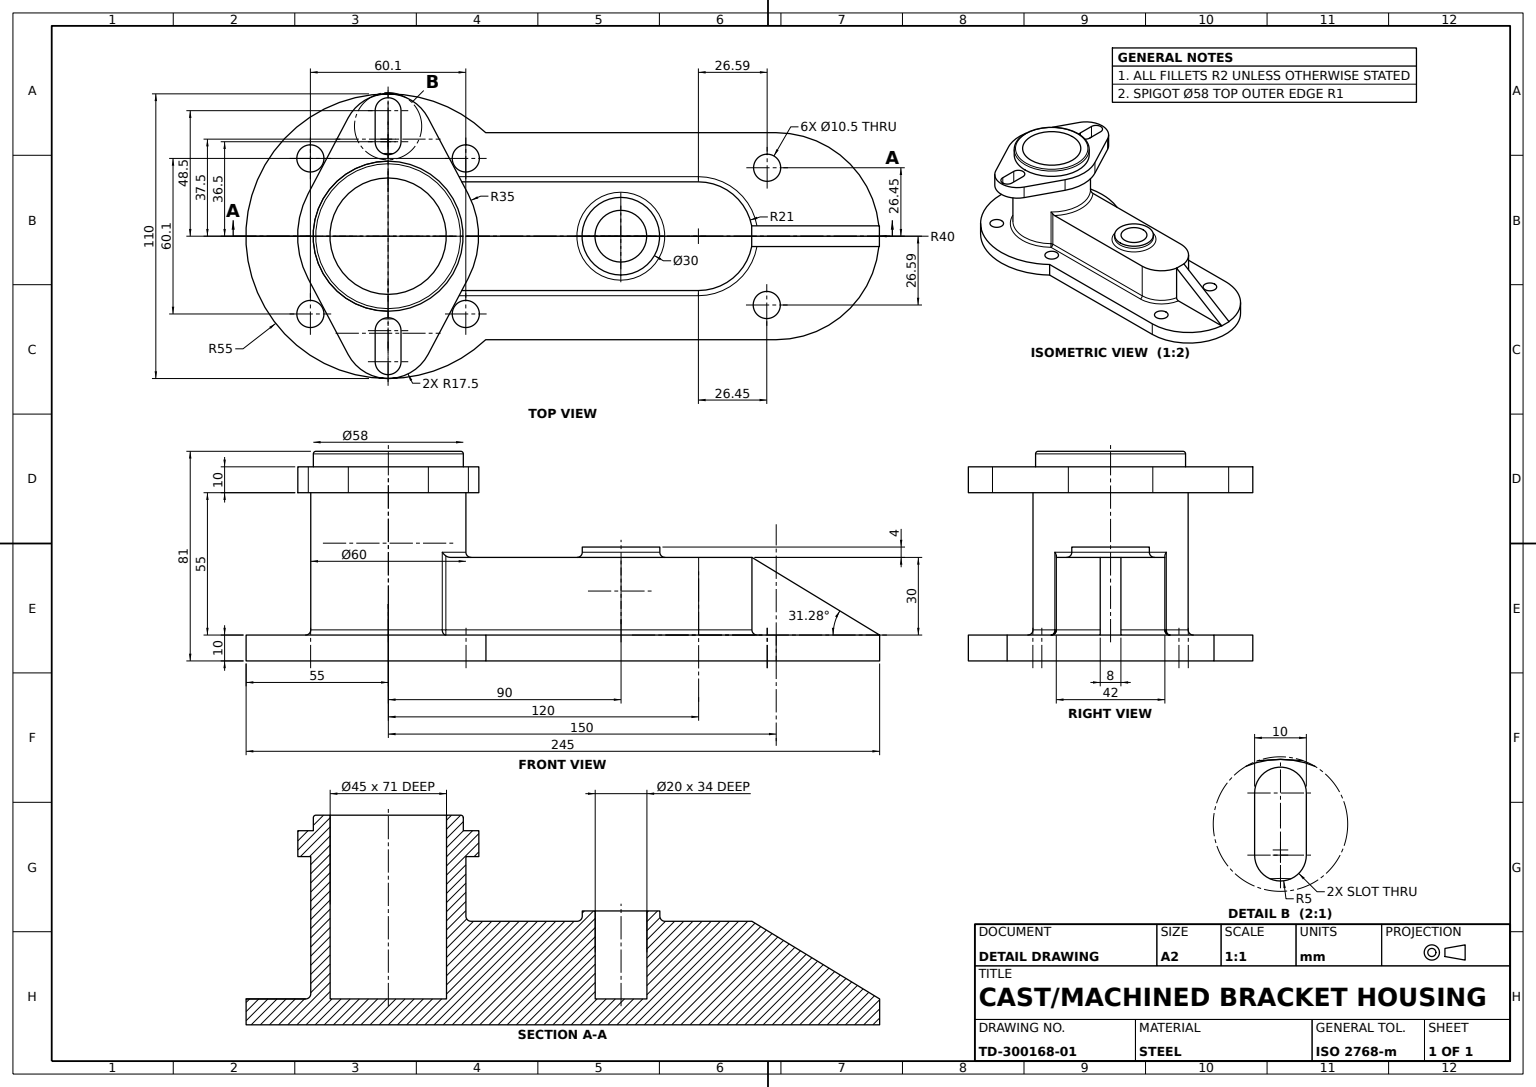
from build123d import *

# Parameters (mm, degrees)
BASE_PLATE_DEPTH                  = 10
BEARING_COLUMN_SKETCH_R           = 30
BEARING_COLUMN_60_DEPTH           = 55
TOP_FLANGE_DEPTH                  = 10
BEARING_SPIGOT_SKETCH_R           = 29
BEARING_SPIGOT_58_DEPTH           = 6
BEARING_BORE_SKETCH_R             = 22.5
BEARING_BORE_45_DEPTH             = 61
FLANGE_SLOTS_2X_DEPTH             = 10
ARM_BLOCK_DEPTH                   = 30
COLUMN_CLEARANCE_SKETCH_R         = 22.5
COLUMN_CLEARANCE_CUT_45_DEPTH     = 30
ARM_BOSS_SKETCH_R                 = 15
ARM_BOSS_30_DEPTH                 = 4
ARM_BOSS_BORE_SKETCH_R            = 10
ARM_BOSS_BORE_20_DEPTH            = 34
BASE_MOUNTING_HOLES_SKETCH_R      = 5.25
BASE_MOUNTING_HOLES_4X_10_5_DEPTH = 34
BASE_DIAGONAL_HOLES_SKETCH_R      = 5.25
BASE_DIAGONAL_HOLES_2X_10_5_DEPTH = 34
GUSSET_RIB_SKETCH_W               = 8
GUSSET_RIB_SKETCH_H               = 30
GUSSET_RIB_DEPTH                  = 50
RIB_TRIM_CUT_DEPTH                = 215.80689002
RIB_TRIM_CUT_DEPTH_BACK           = 49.8
COLUMN_ARM_FILLET_R2_R            = 2
COLUMN_BASE_FILLET_R2_R           = 2
ARM_BOSS_FILLET_R2_R              = 2
SPIGOT_FILLET_R1_R                = 1


with BuildPart() as part:
    # Base Plate Sketch → Base Plate (new body)
    with BuildSketch(Plane(origin=(0, 0, 0), x_dir=(1, 0, 0), z_dir=(0, 1, 0))):
        with BuildLine():
            Line((37.749172176, 40), (150, 40))
            ThreePointArc((150, 40), (190, 0), (150, -40))
            Line((150, -40), (37.749172176, -40))
            ThreePointArc((37.749172176, -40), (-55, 0), (37.749172176, 40))
        make_face()
    extrude(amount=BASE_PLATE_DEPTH)

    # Bearing Column Sketch → Bearing Column Ø60 (add)
    with BuildSketch(Plane(origin=(0, 10, 0), x_dir=(1, 0, 0), z_dir=(0, 1, 0))):
        with Locations(Location((0, 0, 0), (0, 0, 270))):
            Circle(BEARING_COLUMN_SKETCH_R)
    extrude(amount=BEARING_COLUMN_60_DEPTH)

    # Top Flange Sketch → Top Flange (add)
    with BuildSketch(Plane(origin=(0, 65, 0), x_dir=(1, 0, 0), z_dir=(0, 1, 0))):
        with BuildLine():
            Line((-15.477582355, 45.666666667), (-30.95516471, 16.333333333))
            ThreePointArc((-30.95516471, 16.333333333), (-35, 0), (-30.95516471, -16.333333333))
            Line((-30.95516471, -16.333333333), (-15.477582355, -45.666666667))
            ThreePointArc((-15.477582355, -45.666666667), (0, -55), (15.477582355, -45.666666667))
            Line((15.477582355, -45.666666667), (30.95516471, -16.333333333))
            ThreePointArc((30.95516471, -16.333333333), (35, 0), (30.95516471, 16.333333333))
            Line((30.95516471, 16.333333333), (15.477582355, 45.666666667))
            ThreePointArc((15.477582355, 45.666666667), (0, 55), (-15.477582355, 45.666666667))
        make_face()
    extrude(amount=TOP_FLANGE_DEPTH)

    # Bearing Spigot Sketch → Bearing Spigot Ø58 (add)
    with BuildSketch(Plane(origin=(0, 75, 0), x_dir=(1, 0, 0), z_dir=(0, 1, 0))):
        with Locations(Location((0, 0, 0), (0, 0, 270))):
            Circle(BEARING_SPIGOT_SKETCH_R)
    extrude(amount=BEARING_SPIGOT_58_DEPTH)

    # Bearing Bore Sketch → Bearing Bore Ø45 (cut)
    with BuildSketch(Plane(origin=(0, 81, 0), x_dir=(1, 0, 0), z_dir=(0, 1, 0))):
        with Locations(Location((0, 0, 0), (0, 0, 270))):
            Circle(BEARING_BORE_SKETCH_R)
    extrude(amount=-BEARING_BORE_45_DEPTH, mode=Mode.SUBTRACT)

    # Flange Slots Sketch → Flange Slots 2x (cut)
    with BuildSketch(Plane(origin=(0, 75, 0), x_dir=(1, 0, 0), z_dir=(0, 1, 0))):
        with BuildLine():
            Line((-5, 36.5), (-5, 48.5))
            ThreePointArc((-5, 48.5), (0, 53.5), (5, 48.5))
            Line((5, 48.5), (5, 36.5))
            ThreePointArc((5, 36.5), (0, 31.5), (-5, 36.5))
        make_face()
        with BuildLine():
            Line((5, -36.5), (5, -48.5))
            ThreePointArc((5, -48.5), (0, -53.5), (-5, -48.5))
            Line((-5, -48.5), (-5, -36.5))
            ThreePointArc((-5, -36.5), (0, -31.5), (5, -36.5))
        make_face()
    extrude(amount=-FLANGE_SLOTS_2X_DEPTH, mode=Mode.SUBTRACT)

    # Arm Block Sketch → Arm Block (add)
    with BuildSketch(Plane(origin=(0, 10, 0), x_dir=(1, 0, 0), z_dir=(0, 1, 0))):
        with BuildLine():
            Line((120, 21), (20, 21))
            Line((20, 21), (20, -21))
            Line((20, -21), (120, -21))
            ThreePointArc((120, -21), (141, 0), (120, 21))
        make_face()
    extrude(amount=ARM_BLOCK_DEPTH)

    # Column Clearance Sketch → Column Clearance Cut Ø45 (cut)
    with BuildSketch(Plane(origin=(0, 40, 0), x_dir=(1, 0, 0), z_dir=(0, 1, 0))):
        with Locations(Location((0, 0, 0), (0, 0, 270))):
            Circle(COLUMN_CLEARANCE_SKETCH_R)
    extrude(amount=-COLUMN_CLEARANCE_CUT_45_DEPTH, mode=Mode.SUBTRACT)

    # Arm Boss Sketch → Arm Boss Ø30 (add)
    with BuildSketch(Plane(origin=(0, 40, 0), x_dir=(1, 0, 0), z_dir=(0, 1, 0))):
        with Locations(Location((90, 0, 0), (0, 0, 270))):
            Circle(ARM_BOSS_SKETCH_R)
    extrude(amount=ARM_BOSS_30_DEPTH)

    # Arm Boss Bore Sketch → Arm Boss Bore Ø20 (cut)
    with BuildSketch(Plane(origin=(0, 44, 0), x_dir=(1, 0, 0), z_dir=(0, 1, 0))):
        with Locations(Location((90, 0, 0), (0, 0, 270))):
            Circle(ARM_BOSS_BORE_SKETCH_R)
    extrude(amount=-ARM_BOSS_BORE_20_DEPTH, mode=Mode.SUBTRACT)

    # Base Mounting Holes Sketch → Base Mounting Holes 4xØ10.5 (cut)
    with BuildSketch(Plane(origin=(0, 10, 0), x_dir=(1, 0, 0), z_dir=(0, 1, 0))):
        with Locations(Location((-30.0520382, 30.0520382, 0), (0, 0, 270))):
            Circle(BASE_MOUNTING_HOLES_SKETCH_R)
        with Locations(Location((30.0520382, 30.0520382, 0), (0, 0, 270))):
            Circle(BASE_MOUNTING_HOLES_SKETCH_R)
        with Locations(Location((30.0520382, -30.0520382, 0), (0, 0, 270))):
            Circle(BASE_MOUNTING_HOLES_SKETCH_R)
        with Locations(Location((-30.0520382, -30.0520382, 0), (0, 0, 270))):
            Circle(BASE_MOUNTING_HOLES_SKETCH_R)
    extrude(amount=-BASE_MOUNTING_HOLES_4X_10_5_DEPTH, mode=Mode.SUBTRACT)

    # Base Diagonal Holes Sketch → Base Diagonal Holes 2xØ10.5 (cut)
    with BuildSketch(Plane(origin=(0, 10, 0), x_dir=(1, 0, 0), z_dir=(0, 1, 0))):
        with Locations(Location((146.586838162, 26.445983372, 0), (0, 0, 270))):
            Circle(BASE_DIAGONAL_HOLES_SKETCH_R)
        with Locations(Location((146.445983372, -26.586838162, 0), (0, 0, 270))):
            Circle(BASE_DIAGONAL_HOLES_SKETCH_R)
    extrude(amount=-BASE_DIAGONAL_HOLES_2X_10_5_DEPTH, mode=Mode.SUBTRACT)

    # Gusset Rib Sketch → Gusset Rib (add)
    with BuildSketch(Plane(origin=(140, 0, 0), x_dir=(0, 0, -1), z_dir=(1, 0, 0))):
        with Locations((0, 25)):
            Rectangle(GUSSET_RIB_SKETCH_W, GUSSET_RIB_SKETCH_H)
    extrude(amount=GUSSET_RIB_DEPTH)

    # Rib Trim Sketch → Rib Trim Cut (cut, two sides: drawn at the far end of the back side and taken through both)
    with BuildSketch(Plane.XY.offset(4).offset(-RIB_TRIM_CUT_DEPTH_BACK)):
        Polygon((-303.945207186, 310.061044573), (140.615528128, 40), (190, 10), (634.560735315, -260.061044573), (1174.682824461, 629.060426056), (236.17688196, 1199.182515203), align=None)
    extrude(amount=RIB_TRIM_CUT_DEPTH + RIB_TRIM_CUT_DEPTH_BACK, mode=Mode.SUBTRACT)

    # Column-Arm Fillet R2
    column_arm_fillet_r2_edges = [part.edges().sort_by_distance(p)[0] for p in [
        (21.424285286, 25, 21),
        (21.424285286, 25, -21),
        (30, 40, 0),
    ]]
    fillet(column_arm_fillet_r2_edges, radius=COLUMN_ARM_FILLET_R2_R)

    # Column-Base Fillet R2
    column_base_fillet_r2_edges = [part.edges().sort_by_distance(p)[0] for p in [
        (133.360389216, 10, -16.201851746),
        (71.124297731, 10, 21),
        (-27.810744327, 10, -11.25),
        (21.498595461, 10, -21.145950378),
        (21.498595461, 10, 21.145950378),
        (71.124297731, 10, -21),
        (133.360389216, 10, 16.201851746),
    ]]
    fillet(column_base_fillet_r2_edges, radius=COLUMN_BASE_FILLET_R2_R)

    # Arm Boss Fillet R2
    arm_boss_fillet_r2_edges = [part.edges().sort_by_distance(p)[0] for p in [
        (90, 40, -15),
    ]]
    fillet(arm_boss_fillet_r2_edges, radius=ARM_BOSS_FILLET_R2_R)

    # Spigot Fillet R1
    spigot_fillet_r1_edges = [part.edges().sort_by_distance(p)[0] for p in [
        (0, 81, -29),
    ]]
    fillet(spigot_fillet_r1_edges, radius=SPIGOT_FILLET_R1_R)


solid = part.part
